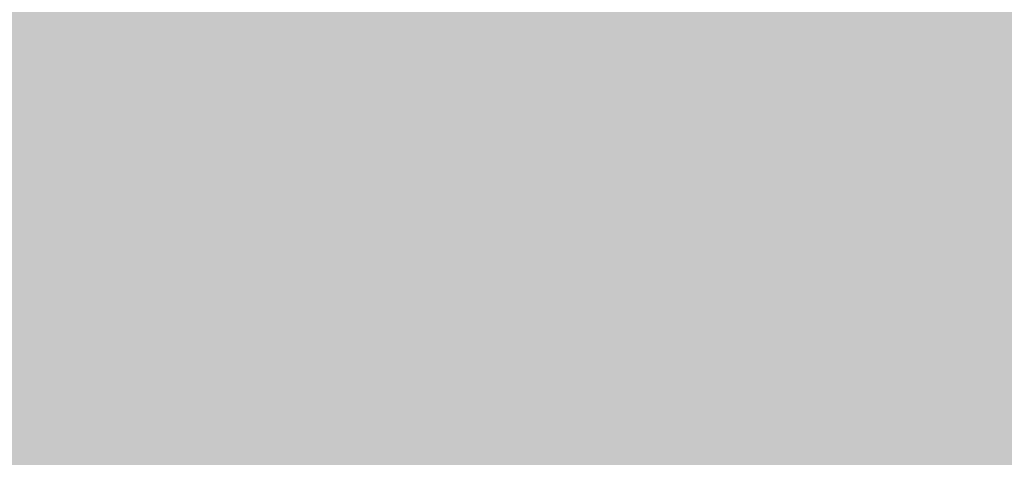
# Model space of a CAD drawing. Units: millimetres. Extents: x 0 to 2267, y 0 to 1823.
# Tile 144 of 256: x 1823.16 to 1833.61, y 1112.67 to 1117.32. Entities that reach past the tile are written whole.
import ezdxf

# ---------------------------------------------------------------- set-up
doc = ezdxf.new("R2010")
doc.units = ezdxf.units.MM
doc.header["$MEASUREMENT"] = 0
doc.layers.add('M-DIMS', color=2, linetype='Continuous', lineweight=25)
doc.layers.add('M-HATC', color=252, linetype='Continuous', lineweight=18)
doc.styles.get("Standard").update_dxf_attribs({"font": 'arial.ttf'})
doc.dimstyles.get("Standard").update_dxf_attribs({"dimtxt": 7, "dimasz": 4, "dimexe": 0.18, "dimexo": 0.0625, "dimgap": 0.09, "dimtad": 0, "dimdec": 0, "dimzin": 0, "dimdsep": 46, "dimtxsty": 'Standard', "dimcen": 0.09, "dimadec": 0, "dimazin": 0, "dimtfac": 1, "dimtdec": 0, "dimtofl": 0, "dimtmove": 0, "dimatfit": 3, "dimfxl": 1, "dimtolj": 1, "dimtzin": 0, "dimarcsym": 0})

# ---------------------------------------------------------------- blocks, each defined once
blk = doc.blocks.new('*D1')
at = {"layer": 'Defpoints', "color": 0, "transparency": 16777216}
for p in [(1593.429, 1127.417), (1843.429, 1127.417), (1843.429, 955.628)]:
    blk.add_point(p, dxfattribs=at)
at = {"layer": 'M-DIMS', "color": 0, "lineweight": -2, "transparency": 16777216}
for p, q in [((1593.429, 1127.355), (1593.429, 955.448)), ((1843.429, 1127.355), (1843.429, 955.448)), ((1597.429, 955.628), (1710.558, 955.628)), ((1839.429, 955.628), (1726.3, 955.628))]:
    blk.add_line(p, q, dxfattribs=at)
at = {"layer": 'M-DIMS', "color": 0, "transparency": 16777216}
for points in [[(1597.429, 956.294), (1597.429, 954.961), (1593.429, 955.628)], [(1839.429, 956.294), (1839.429, 954.961), (1843.429, 955.628)]]:
    blk.add_solid(points, dxfattribs=at)
at = {"layer": 'M-DIMS', "color": 0, "transparency": 16777216, "insert": (1718.429, 955.628), "char_height": 7, "attachment_point": 5}
blk.add_mtext('\\A1;250', dxfattribs=at)

msp = doc.modelspace()

# ---------------------------------------------------------------- hatches: boundary and pattern name
at = {"layer": 'M-HATC'}
h = msp.add_hatch(color=256, dxfattribs=at)
h.dxf.hatch_style = 1
h.paths.add_polyline_path([(2065.771, 1618.062, 0.236068), (2055.771, 1638.062), (1381.087, 1638.062, 0.236068), (1371.087, 1618.062), (1371.087, 1603.062), (2055.771, 1603.062), (2065.771, 1603.062)])
h.paths.add_polyline_path([(2062.772, 1550.296), (2062.772, 1560.296), (1374.086, 1560.296), (1374.086, 1550.296), (1374.086, 1540.296), (1384.086, 1540.296), (1389.086, 1540.296), (2062.772, 1540.296)])
h.paths.add_polyline_path([(1930.929, 1282.766), (1505.929, 1282.766), (1587.628, 1235.597, 0.131652), (1600.128, 1232.247), (1836.73, 1232.247, 0.131652), (1849.23, 1235.597)])
h.paths.add_polyline_path([(1930.929, 1117.417), (1905.929, 1117.417), (1505.929, 1117.417), (1505.929, 1077.417), (1930.929, 1077.417)])

# ---------------------------------------------------------------- dimensions: what is measured, and where the dimension line sits
at = {"layer": 'M-DIMS'}
dim = msp.add_linear_dim(base=(1843.429, 955.628), p1=(1593.429, 1127.417), p2=(1843.429, 1127.417), dimstyle='Standard', override={"dimclrd": 0, "dimclre": 0, "dimclrt": 0}, dxfattribs=at)
dim.commit()
dim.dimension.update_dxf_attribs({"geometry": '*D1', "text_midpoint": (1718.429, 955.628)})

doc.saveas('drawing.dxf')
